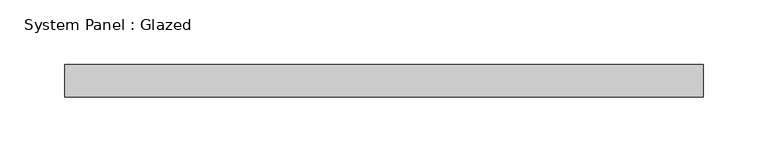
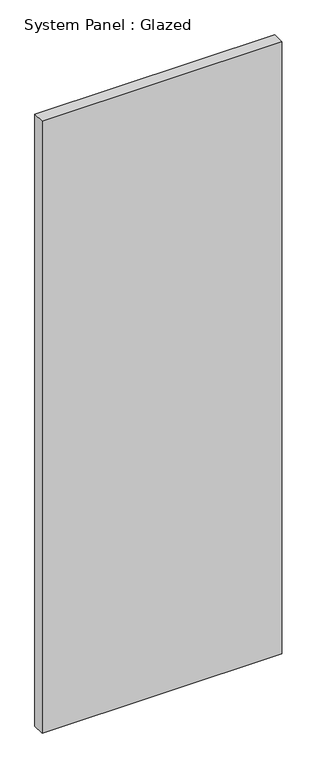
"""IFC4 building model written with IfcOpenShell, lengths in millimetres: plate geometry, System Panel : Glazed."""

from ifc_helpers import new_model, si_unit, origin, origin_with_axes, place, context, project, spatial, polyline, outline, extrude, source, transform, mapped, element, save


def system_panel_glazed_13fbf6b0(model_context):
    return source(origin(), model_context, "Body", "SweptSolid", [
        extrude(outline(polyline([(247.65, 19.05), (-247.65, 19.05), (-247.65, 44.45), (247.65, 44.45), (247.65, 19.05)])), origin_with_axes(), (0.0, 0.0, 1.0), 1335.4986146),
    ])


if __name__ == "__main__":
    model = new_model("IFC4")
    model_context = context("Model", 3, world=origin())
    ifc_project = project(units=[si_unit("LENGTHUNIT", "METRE", prefix="MILLI")], contexts=[model_context])
    site = spatial("IfcSite", under=ifc_project)
    building = spatial("IfcBuilding", under=site)
    placement = place(None, origin())
    system_panel_glazed_shape = system_panel_glazed_13fbf6b0(model_context)
    element("IfcPlate", 1, ObjectType="System Panel : Glazed", at=placement, inside=building, context=model_context, shape_type="MappedRepresentation", body=[
        mapped(system_panel_glazed_shape, transform((0.0, 0.0, 0.0), x_axis=(1.0, 0.0, 0.0), y_axis=(0.0, 1.0, 0.0), z_axis=(0.0, 0.0, 1.0))),
    ])
    save(model, "model.ifc")

# Revit data of these elements
# Type "System Panel : Glazed"
#   Construction Type Id = "GSP4R"
#   Analytic Construction = "1/8 in Pilkington single glazing"
#   Visual Light Transmittance = 0.9
#   Solar Heat Gain Coefficient = 0.86
#   Heat Transfer Coefficient (U) = 1.18115 BTU/(h·ft²·°F)
#   Define Thermal Properties by = 1
# Element 1 (IfcPlate, "System Panel : Glazed")
#   Materials on its faces: "Glass"
# Materials
#   "Glass": class "Glass", colour RGB 0 128 192, transparency 0.75, Description = "Soda Lime Glass", Cost = 0
